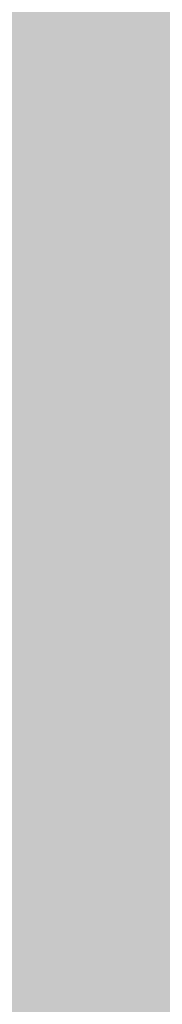
# Model space of a CAD drawing. Units: millimetres. Extents: x -22994 to 29398, y -19990 to 20176.
# Tile 80 of 135: x 225.543 to 225.814, y 85.199 to 87.071. Entities that reach past the tile are written whole.
import ezdxf
from ezdxf import colors
from ezdxf.entities.mleader import LeaderData, LeaderLine
from ezdxf.math import Vec2, Vec3

# ---------------------------------------------------------------- set-up
doc = ezdxf.new("R2010")
doc.units = ezdxf.units.MM
doc.header["$MEASUREMENT"] = 0
doc.layers.add('M-ANNO-TEXT', color=7, linetype='Continuous', lineweight=25)
doc.layers.add('M-DIMS', color=2, linetype='Continuous', lineweight=18)
doc.styles.get("Standard").update_dxf_attribs({"font": 'arial.ttf'})
doc.dimstyles.get("Standard").update_dxf_attribs({"dimtxt": 0.18, "dimasz": 10000, "dimexe": 0.18, "dimexo": 0.0625, "dimgap": 0.09, "dimtad": 0, "dimtih": 1, "dimtoh": 1, "dimdec": 0, "dimzin": 0, "dimdsep": 46, "dimtxsty": 'Standard', "dimcen": 0.09, "dimadec": 0, "dimazin": 0, "dimtfac": 1, "dimtdec": 0, "dimtofl": 0, "dimtmove": 0, "dimatfit": 3, "dimfxl": 1, "dimtolj": 1, "dimtzin": 0, "dimlwd": 30, "dimarcsym": 0})

# ---------------------------------------------------------------- blocks, each defined once
blk = doc.blocks.new('*D2')
at = {"layer": 'Defpoints', "color": 0, "transparency": 16777216}
for p in [(6.6773, 10.2713), (290.852, 10.2713), (290.852, -5.0787)]:
    blk.add_point(p, dxfattribs=at)
at = {"layer": 'M-DIMS', "color": 0, "lineweight": -2, "transparency": 16777216}
for p, q in [((6.6773, 10.2088), (6.6773, -5.2587)), ((290.852, 10.2088), (290.852, -5.2587))]:
    blk.add_line(p, q, dxfattribs=at)
at = {"layer": 'M-DIMS', "color": 0, "lineweight": 30, "transparency": 16777216}
for p, q in [((-9993.3227, -5.0787), (-19993.3227, -5.0787)), ((10290.852, -5.0787), (20290.852, -5.0787))]:
    blk.add_line(p, q, dxfattribs=at)
at = {"layer": 'M-DIMS', "color": 0, "transparency": 16777216}
for points in [[(-9993.3227, 1661.5879), (-9993.3227, -1671.7454), (6.6773, -5.0787)], [(10290.852, 1661.5879), (10290.852, -1671.7454), (290.852, -5.0787)]]:
    blk.add_solid(points, dxfattribs=at)
at = {"layer": 'M-DIMS', "color": 0, "transparency": 16777216, "insert": (148.7647, -5.0787), "char_height": 0.18, "attachment_point": 5}
blk.add_mtext('\\A1;284.2', dxfattribs=at)
blk = doc.blocks.new('*D3')
at = {"layer": 'Defpoints', "color": 0, "transparency": 16777216}
for p in [(110.2647, 204.1654), (110.2647, 176.3662), (95.8327, 127.967)]:
    blk.add_point(p, dxfattribs=at)
at = {"layer": 'M-DIMS', "color": 0, "lineweight": -2, "transparency": 16777216}
for p, q in [((95.8327, 128.0295), (95.8327, 204.3454)), ((110.2647, 176.4287), (110.2647, 204.3454))]:
    blk.add_line(p, q, dxfattribs=at)
at = {"layer": 'M-DIMS', "color": 0, "lineweight": 30, "transparency": 16777216}
for p, q in [((-9904.1673, 204.1654), (-19904.1673, 204.1654)), ((10110.2647, 204.1654), (20110.2647, 204.1654))]:
    blk.add_line(p, q, dxfattribs=at)
at = {"layer": 'M-DIMS', "color": 0, "transparency": 16777216}
for points in [[(-9904.1673, 1870.8321), (-9904.1673, -1462.5013), (95.8327, 204.1654)], [(10110.2647, 1870.8321), (10110.2647, -1462.5013), (110.2647, 204.1654)]]:
    blk.add_solid(points, dxfattribs=at)
at = {"layer": 'M-DIMS', "color": 0, "transparency": 16777216, "insert": (103.0487, 204.1654), "char_height": 0.18, "attachment_point": 5}
blk.add_mtext('\\A1;14.432', dxfattribs=at)
blk = doc.blocks.new('*D4')
at = {"layer": 'Defpoints', "color": 0, "transparency": 16777216}
for p in [(116.2647, 204.1654), (110.2647, 176.3662), (116.2647, 176.3662)]:
    blk.add_point(p, dxfattribs=at)
at = {"layer": 'M-DIMS', "color": 0, "lineweight": -2, "transparency": 16777216}
for p, q in [((110.2647, 176.4287), (110.2647, 204.3454)), ((116.2647, 176.4287), (116.2647, 204.3454))]:
    blk.add_line(p, q, dxfattribs=at)
at = {"layer": 'M-DIMS', "color": 0, "lineweight": 30, "transparency": 16777216}
for p, q in [((-9889.7353, 204.1654), (-19889.7353, 204.1654)), ((10116.2647, 204.1654), (20116.2647, 204.1654))]:
    blk.add_line(p, q, dxfattribs=at)
at = {"layer": 'M-DIMS', "color": 0, "transparency": 16777216}
for points in [[(-9889.7353, 1870.8321), (-9889.7353, -1462.5013), (110.2647, 204.1654)], [(10116.2647, 1870.8321), (10116.2647, -1462.5013), (116.2647, 204.1654)]]:
    blk.add_solid(points, dxfattribs=at)
at = {"layer": 'M-DIMS', "color": 0, "transparency": 16777216, "insert": (113.2647, 204.1654), "char_height": 0.18, "attachment_point": 5}
blk.add_mtext('\\A1;6', dxfattribs=at)
blk = doc.blocks.new('*D5')
at = {"layer": 'Defpoints', "color": 0, "transparency": 16777216}
for p in [(181.2647, 204.1654), (116.2647, 176.3662), (181.2647, 176.3662)]:
    blk.add_point(p, dxfattribs=at)
at = {"layer": 'M-DIMS', "color": 0, "lineweight": -2, "transparency": 16777216}
for p, q in [((116.2647, 176.4287), (116.2647, 204.3454)), ((181.2647, 176.4287), (181.2647, 204.3454))]:
    blk.add_line(p, q, dxfattribs=at)
at = {"layer": 'M-DIMS', "color": 0, "lineweight": 30, "transparency": 16777216}
for p, q in [((-9883.7353, 204.1654), (-19883.7353, 204.1654)), ((10181.2647, 204.1654), (20181.2647, 204.1654))]:
    blk.add_line(p, q, dxfattribs=at)
at = {"layer": 'M-DIMS', "color": 0, "transparency": 16777216}
for points in [[(-9883.7353, 1870.8321), (-9883.7353, -1462.5013), (116.2647, 204.1654)], [(10181.2647, 1870.8321), (10181.2647, -1462.5013), (181.2647, 204.1654)]]:
    blk.add_solid(points, dxfattribs=at)
at = {"layer": 'M-DIMS', "color": 0, "transparency": 16777216, "insert": (148.7647, 204.1654), "char_height": 0.18, "attachment_point": 5}
blk.add_mtext('\\A1;65', dxfattribs=at)
blk = doc.blocks.new('*D6')
at = {"layer": 'Defpoints', "color": 0, "transparency": 16777216}
for p in [(187.2647, 204.1654), (181.2647, 176.3662), (187.2647, 176.3662)]:
    blk.add_point(p, dxfattribs=at)
at = {"layer": 'M-DIMS', "color": 0, "lineweight": -2, "transparency": 16777216}
for p, q in [((181.2647, 176.4287), (181.2647, 204.3454)), ((187.2647, 176.4287), (187.2647, 204.3454))]:
    blk.add_line(p, q, dxfattribs=at)
at = {"layer": 'M-DIMS', "color": 0, "lineweight": 30, "transparency": 16777216}
for p, q in [((-9818.7353, 204.1654), (-19818.7353, 204.1654)), ((10187.2647, 204.1654), (20187.2647, 204.1654))]:
    blk.add_line(p, q, dxfattribs=at)
at = {"layer": 'M-DIMS', "color": 0, "transparency": 16777216}
for points in [[(-9818.7353, 1870.8321), (-9818.7353, -1462.5013), (181.2647, 204.1654)], [(10187.2647, 1870.8321), (10187.2647, -1462.5013), (187.2647, 204.1654)]]:
    blk.add_solid(points, dxfattribs=at)
at = {"layer": 'M-DIMS', "color": 0, "transparency": 16777216, "insert": (184.2647, 204.1654), "char_height": 0.18, "attachment_point": 5}
blk.add_mtext('\\A1;6', dxfattribs=at)
blk = doc.blocks.new('*D7')
at = {"layer": 'Defpoints', "color": 0, "transparency": 16777216}
for p in [(201.6967, 204.1654), (187.2647, 176.3662), (201.6967, 127.967)]:
    blk.add_point(p, dxfattribs=at)
at = {"layer": 'M-DIMS', "color": 0, "lineweight": -2, "transparency": 16777216}
for p, q in [((187.2647, 176.4287), (187.2647, 204.3454)), ((201.6967, 128.0295), (201.6967, 204.3454))]:
    blk.add_line(p, q, dxfattribs=at)
at = {"layer": 'M-DIMS', "color": 0, "lineweight": 30, "transparency": 16777216}
for p, q in [((-9812.7353, 204.1654), (-19812.7353, 204.1654)), ((10201.6967, 204.1654), (20201.6967, 204.1654))]:
    blk.add_line(p, q, dxfattribs=at)
at = {"layer": 'M-DIMS', "color": 0, "transparency": 16777216}
for points in [[(-9812.7353, 1870.8321), (-9812.7353, -1462.5013), (187.2647, 204.1654)], [(10201.6967, 1870.8321), (10201.6967, -1462.5013), (201.6967, 204.1654)]]:
    blk.add_solid(points, dxfattribs=at)
at = {"layer": 'M-DIMS', "color": 0, "transparency": 16777216, "insert": (194.4807, 204.1654), "char_height": 0.18, "attachment_point": 5}
blk.add_mtext('\\A1;14.432', dxfattribs=at)
blk = doc.blocks.new('*D8')
at = {"layer": 'Defpoints', "color": 0, "transparency": 16777216}
for p in [(227.6485, 204.1654), (227.6485, 146.7296), (201.6967, 127.967)]:
    blk.add_point(p, dxfattribs=at)
at = {"layer": 'M-DIMS', "color": 0, "lineweight": -2, "transparency": 16777216}
for p, q in [((201.6967, 128.0295), (201.6967, 204.3454)), ((227.6485, 146.7921), (227.6485, 204.3454))]:
    blk.add_line(p, q, dxfattribs=at)
at = {"layer": 'M-DIMS', "color": 0, "lineweight": 30, "transparency": 16777216}
for p, q in [((-9798.3033, 204.1654), (-19798.3033, 204.1654)), ((10227.6485, 204.1654), (20227.6485, 204.1654))]:
    blk.add_line(p, q, dxfattribs=at)
at = {"layer": 'M-DIMS', "color": 0, "transparency": 16777216}
for points in [[(-9798.3033, 1870.8321), (-9798.3033, -1462.5013), (201.6967, 204.1654)], [(10227.6485, 1870.8321), (10227.6485, -1462.5013), (227.6485, 204.1654)]]:
    blk.add_solid(points, dxfattribs=at)
at = {"layer": 'M-DIMS', "color": 0, "transparency": 16777216, "insert": (214.6726, 204.1654), "char_height": 0.18, "attachment_point": 5}
blk.add_mtext('\\A1;25.95', dxfattribs=at)
blk = doc.blocks.new('*D9')
at = {"layer": 'Defpoints', "color": 0, "transparency": 16777216}
for p in [(187.2647, 176.3662), (306.202, 176.3662), (290.852, 10.2713)]:
    blk.add_point(p, dxfattribs=at)
at = {"layer": 'M-DIMS', "color": 0, "lineweight": 30, "transparency": 16777216}
for p, q in [((306.202, 10176.3662), (306.202, 20176.3662)), ((306.202, -9989.7287), (306.202, -19989.7287))]:
    blk.add_line(p, q, dxfattribs=at)
at = {"layer": 'M-DIMS', "color": 0, "lineweight": -2, "transparency": 16777216}
for p, q in [((187.3272, 176.3662), (306.382, 176.3662)), ((290.9145, 10.2713), (306.382, 10.2713))]:
    blk.add_line(p, q, dxfattribs=at)
at = {"layer": 'M-DIMS', "color": 0, "transparency": 16777216}
for points in [[(-1360.4646, 10176.3662), (1972.8687, 10176.3662), (306.202, 176.3662)], [(-1360.4646, -9989.7287), (1972.8687, -9989.7287), (306.202, 10.2713)]]:
    blk.add_solid(points, dxfattribs=at)
at = {"layer": 'M-DIMS', "color": 0, "transparency": 16777216, "insert": (306.202, 93.3187), "char_height": 0.18, "attachment_point": 5}
blk.add_mtext('\\A1;166.1', dxfattribs=at)
blk = doc.blocks.new('*D10')
at = {"layer": 'Defpoints', "color": 0, "transparency": 16777216}
for p in [(125.6498, 136.0713), (133.3459, 136.0713), (133.3459, -5.0787)]:
    blk.add_point(p, dxfattribs=at)
at = {"layer": 'M-DIMS', "color": 0, "lineweight": -2, "transparency": 16777216}
for p, q in [((125.6498, 136.0088), (125.6498, -5.2587)), ((133.3459, 136.0088), (133.3459, -5.2587))]:
    blk.add_line(p, q, dxfattribs=at)
at = {"layer": 'M-DIMS', "color": 0, "lineweight": 30, "transparency": 16777216}
for p, q in [((-9874.3502, -5.0787), (-19874.3502, -5.0787)), ((10133.3459, -5.0787), (20133.3459, -5.0787))]:
    blk.add_line(p, q, dxfattribs=at)
at = {"layer": 'M-DIMS', "color": 0, "transparency": 16777216}
for points in [[(-9874.3502, 1661.5879), (-9874.3502, -1671.7454), (125.6498, -5.0787)], [(10133.3459, 1661.5879), (10133.3459, -1671.7454), (133.3459, -5.0787)]]:
    blk.add_solid(points, dxfattribs=at)
at = {"layer": 'M-DIMS', "color": 0, "transparency": 16777216, "insert": (129.4978, -5.0787), "char_height": 0.18, "attachment_point": 5}
blk.add_mtext('\\A1;7.696', dxfattribs=at)
blk = doc.blocks.new('*D11')
at = {"layer": 'Defpoints', "color": 0, "transparency": 16777216}
for p in [(133.3459, 136.0713), (135.6498, 136.0713), (135.6498, -5.0787)]:
    blk.add_point(p, dxfattribs=at)
at = {"layer": 'M-DIMS', "color": 0, "lineweight": -2, "transparency": 16777216}
for p, q in [((133.3459, 136.0088), (133.3459, -5.2587)), ((135.6498, 136.0088), (135.6498, -5.2587))]:
    blk.add_line(p, q, dxfattribs=at)
at = {"layer": 'M-DIMS', "color": 0, "lineweight": 30, "transparency": 16777216}
for p, q in [((-9866.6541, -5.0787), (-19866.6541, -5.0787)), ((10135.6498, -5.0787), (20135.6498, -5.0787))]:
    blk.add_line(p, q, dxfattribs=at)
at = {"layer": 'M-DIMS', "color": 0, "transparency": 16777216}
for points in [[(-9866.6541, 1661.5879), (-9866.6541, -1671.7454), (133.3459, -5.0787)], [(10135.6498, 1661.5879), (10135.6498, -1671.7454), (135.6498, -5.0787)]]:
    blk.add_solid(points, dxfattribs=at)
at = {"layer": 'M-DIMS', "color": 0, "transparency": 16777216, "insert": (134.4978, -5.0787), "char_height": 0.18, "attachment_point": 5}
blk.add_mtext('\\A1;2.304', dxfattribs=at)
blk = doc.blocks.new('*D12')
at = {"layer": 'Defpoints', "color": 0, "transparency": 16777216}
for p in [(135.6498, 136.0713), (145.6498, 136.0713), (145.6498, -5.0787)]:
    blk.add_point(p, dxfattribs=at)
at = {"layer": 'M-DIMS', "color": 0, "lineweight": -2, "transparency": 16777216}
for p, q in [((135.6498, 136.0088), (135.6498, -5.2587)), ((145.6498, 136.0088), (145.6498, -5.2587))]:
    blk.add_line(p, q, dxfattribs=at)
at = {"layer": 'M-DIMS', "color": 0, "lineweight": 30, "transparency": 16777216}
for p, q in [((-9864.3502, -5.0787), (-19864.3502, -5.0787)), ((10145.6498, -5.0787), (20145.6498, -5.0787))]:
    blk.add_line(p, q, dxfattribs=at)
at = {"layer": 'M-DIMS', "color": 0, "transparency": 16777216}
for points in [[(-9864.3502, 1661.5879), (-9864.3502, -1671.7454), (135.6498, -5.0787)], [(10145.6498, 1661.5879), (10145.6498, -1671.7454), (145.6498, -5.0787)]]:
    blk.add_solid(points, dxfattribs=at)
at = {"layer": 'M-DIMS', "color": 0, "transparency": 16777216, "insert": (140.6498, -5.0787), "char_height": 0.18, "attachment_point": 5}
blk.add_mtext('\\A1;10', dxfattribs=at)
blk = doc.blocks.new('*D13')
at = {"layer": 'Defpoints', "color": 0, "transparency": 16777216}
for p in [(145.6498, 136.0713), (155.6498, 136.0713), (155.6498, -5.0787)]:
    blk.add_point(p, dxfattribs=at)
at = {"layer": 'M-DIMS', "color": 0, "lineweight": -2, "transparency": 16777216}
for p, q in [((145.6498, 136.0088), (145.6498, -5.2587)), ((155.6498, 136.0088), (155.6498, -5.2587))]:
    blk.add_line(p, q, dxfattribs=at)
at = {"layer": 'M-DIMS', "color": 0, "lineweight": 30, "transparency": 16777216}
for p, q in [((-9854.3502, -5.0787), (-19854.3502, -5.0787)), ((10155.6498, -5.0787), (20155.6498, -5.0787))]:
    blk.add_line(p, q, dxfattribs=at)
at = {"layer": 'M-DIMS', "color": 0, "transparency": 16777216}
for points in [[(-9854.3502, 1661.5879), (-9854.3502, -1671.7454), (145.6498, -5.0787)], [(10155.6498, 1661.5879), (10155.6498, -1671.7454), (155.6498, -5.0787)]]:
    blk.add_solid(points, dxfattribs=at)
at = {"layer": 'M-DIMS', "color": 0, "transparency": 16777216, "insert": (150.6498, -5.0787), "char_height": 0.18, "attachment_point": 5}
blk.add_mtext('\\A1;10', dxfattribs=at)
blk = doc.blocks.new('*D14')
at = {"layer": 'Defpoints', "color": 0, "transparency": 16777216}
for p in [(155.6498, 136.0713), (165.6498, 136.0713), (165.6498, -5.0787)]:
    blk.add_point(p, dxfattribs=at)
at = {"layer": 'M-DIMS', "color": 0, "lineweight": -2, "transparency": 16777216}
for p, q in [((155.6498, 136.0088), (155.6498, -5.2587)), ((165.6498, 136.0088), (165.6498, -5.2587))]:
    blk.add_line(p, q, dxfattribs=at)
at = {"layer": 'M-DIMS', "color": 0, "lineweight": 30, "transparency": 16777216}
for p, q in [((-9844.3502, -5.0787), (-19844.3502, -5.0787)), ((10165.6498, -5.0787), (20165.6498, -5.0787))]:
    blk.add_line(p, q, dxfattribs=at)
at = {"layer": 'M-DIMS', "color": 0, "transparency": 16777216}
for points in [[(-9844.3502, 1661.5879), (-9844.3502, -1671.7454), (155.6498, -5.0787)], [(10165.6498, 1661.5879), (10165.6498, -1671.7454), (165.6498, -5.0787)]]:
    blk.add_solid(points, dxfattribs=at)
at = {"layer": 'M-DIMS', "color": 0, "transparency": 16777216, "insert": (160.6498, -5.0787), "char_height": 0.18, "attachment_point": 5}
blk.add_mtext('\\A1;10', dxfattribs=at)
blk = doc.blocks.new('*D15')
at = {"layer": 'Defpoints', "color": 0, "transparency": 16777216}
for p in [(173.3459, 154.788), (173.3459, 136.0713), (306.202, 136.0713)]:
    blk.add_point(p, dxfattribs=at)
at = {"layer": 'M-DIMS', "color": 0, "lineweight": 30, "transparency": 16777216}
for p, q in [((306.202, 10154.788), (306.202, 20154.788)), ((306.202, -9863.9287), (306.202, -19863.9287))]:
    blk.add_line(p, q, dxfattribs=at)
at = {"layer": 'M-DIMS', "color": 0, "lineweight": -2, "transparency": 16777216}
for p, q in [((173.4084, 154.788), (306.382, 154.788)), ((173.4084, 136.0713), (306.382, 136.0713))]:
    blk.add_line(p, q, dxfattribs=at)
at = {"layer": 'M-DIMS', "color": 0, "transparency": 16777216}
for points in [[(-1360.4646, 10154.788), (1972.8687, 10154.788), (306.202, 154.788)], [(-1360.4646, -9863.9287), (1972.8687, -9863.9287), (306.202, 136.0713)]]:
    blk.add_solid(points, dxfattribs=at)
at = {"layer": 'M-DIMS', "color": 0, "transparency": 16777216, "insert": (306.202, 145.4297), "char_height": 0.18, "attachment_point": 5}
blk.add_mtext('\\A1;18.717', dxfattribs=at)
blk = doc.blocks.new('*D16')
at = {"layer": 'Defpoints', "color": 0, "transparency": 16777216}
for p in [(120.1702, 204.1654), (110.4658, 48.0349), (120.1702, 48.0349)]:
    blk.add_point(p, dxfattribs=at)
at = {"layer": 'M-DIMS', "color": 0, "lineweight": -2, "transparency": 16777216}
for p, q in [((110.4658, 48.0974), (110.4658, 204.3454)), ((120.1702, 48.0974), (120.1702, 204.3454))]:
    blk.add_line(p, q, dxfattribs=at)
at = {"layer": 'M-DIMS', "color": 0, "lineweight": 30, "transparency": 16777216}
for p, q in [((-9889.5342, 204.1654), (-19889.5342, 204.1654)), ((10120.1702, 204.1654), (20120.1702, 204.1654))]:
    blk.add_line(p, q, dxfattribs=at)
at = {"layer": 'M-DIMS', "color": 0, "transparency": 16777216}
for points in [[(-9889.5342, 1870.8321), (-9889.5342, -1462.5013), (110.4658, 204.1654)], [(10120.1702, 1870.8321), (10120.1702, -1462.5013), (120.1702, 204.1654)]]:
    blk.add_solid(points, dxfattribs=at)
at = {"layer": 'M-DIMS', "color": 0, "transparency": 16777216, "insert": (115.318, 204.1654), "char_height": 0.18, "attachment_point": 5}
blk.add_mtext('\\A1;9.704', dxfattribs=at)
blk = doc.blocks.new('*D17')
at = {"layer": 'Defpoints', "color": 0, "transparency": 16777216}
for p in [(126.1702, 204.1654), (120.1702, 48.0349), (126.1702, 48.0349)]:
    blk.add_point(p, dxfattribs=at)
at = {"layer": 'M-DIMS', "color": 0, "lineweight": -2, "transparency": 16777216}
for p, q in [((120.1702, 48.0974), (120.1702, 204.3454)), ((126.1702, 48.0974), (126.1702, 204.3454))]:
    blk.add_line(p, q, dxfattribs=at)
at = {"layer": 'M-DIMS', "color": 0, "lineweight": 30, "transparency": 16777216}
for p, q in [((-9879.8298, 204.1654), (-19879.8298, 204.1654)), ((10126.1702, 204.1654), (20126.1702, 204.1654))]:
    blk.add_line(p, q, dxfattribs=at)
at = {"layer": 'M-DIMS', "color": 0, "transparency": 16777216}
for points in [[(-9879.8298, 1870.8321), (-9879.8298, -1462.5013), (120.1702, 204.1654)], [(10126.1702, 1870.8321), (10126.1702, -1462.5013), (126.1702, 204.1654)]]:
    blk.add_solid(points, dxfattribs=at)
at = {"layer": 'M-DIMS', "color": 0, "transparency": 16777216, "insert": (123.1702, 204.1654), "char_height": 0.18, "attachment_point": 5}
blk.add_mtext('\\A1;6', dxfattribs=at)
blk = doc.blocks.new('*D18')
at = {"layer": 'Defpoints', "color": 0, "transparency": 16777216}
for p in [(132.1702, 204.1654), (126.1702, 48.0349), (132.1702, 48.0349)]:
    blk.add_point(p, dxfattribs=at)
at = {"layer": 'M-DIMS', "color": 0, "lineweight": -2, "transparency": 16777216}
for p, q in [((126.1702, 48.0974), (126.1702, 204.3454)), ((132.1702, 48.0974), (132.1702, 204.3454))]:
    blk.add_line(p, q, dxfattribs=at)
at = {"layer": 'M-DIMS', "color": 0, "lineweight": 30, "transparency": 16777216}
for p, q in [((-9873.8298, 204.1654), (-19873.8298, 204.1654)), ((10132.1702, 204.1654), (20132.1702, 204.1654))]:
    blk.add_line(p, q, dxfattribs=at)
at = {"layer": 'M-DIMS', "color": 0, "transparency": 16777216}
for points in [[(-9873.8298, 1870.8321), (-9873.8298, -1462.5013), (126.1702, 204.1654)], [(10132.1702, 1870.8321), (10132.1702, -1462.5013), (132.1702, 204.1654)]]:
    blk.add_solid(points, dxfattribs=at)
at = {"layer": 'M-DIMS', "color": 0, "transparency": 16777216, "insert": (129.1702, 204.1654), "char_height": 0.18, "attachment_point": 5}
blk.add_mtext('\\A1;6', dxfattribs=at)
blk = doc.blocks.new('*D19')
at = {"layer": 'Defpoints', "color": 0, "transparency": 16777216}
for p in [(138.1702, 204.1654), (132.1702, 48.0349), (138.1702, 48.0349)]:
    blk.add_point(p, dxfattribs=at)
at = {"layer": 'M-DIMS', "color": 0, "lineweight": -2, "transparency": 16777216}
for p, q in [((132.1702, 48.0974), (132.1702, 204.3454)), ((138.1702, 48.0974), (138.1702, 204.3454))]:
    blk.add_line(p, q, dxfattribs=at)
at = {"layer": 'M-DIMS', "color": 0, "lineweight": 30, "transparency": 16777216}
for p, q in [((-9867.8298, 204.1654), (-19867.8298, 204.1654)), ((10138.1702, 204.1654), (20138.1702, 204.1654))]:
    blk.add_line(p, q, dxfattribs=at)
at = {"layer": 'M-DIMS', "color": 0, "transparency": 16777216}
for points in [[(-9867.8298, 1870.8321), (-9867.8298, -1462.5013), (132.1702, 204.1654)], [(10138.1702, 1870.8321), (10138.1702, -1462.5013), (138.1702, 204.1654)]]:
    blk.add_solid(points, dxfattribs=at)
at = {"layer": 'M-DIMS', "color": 0, "transparency": 16777216, "insert": (135.1702, 204.1654), "char_height": 0.18, "attachment_point": 5}
blk.add_mtext('\\A1;6', dxfattribs=at)
blk = doc.blocks.new('*D20')
at = {"layer": 'Defpoints', "color": 0, "transparency": 16777216}
for p in [(144.1702, 204.1654), (138.1702, 48.0349), (144.1702, 48.0349)]:
    blk.add_point(p, dxfattribs=at)
at = {"layer": 'M-DIMS', "color": 0, "lineweight": -2, "transparency": 16777216}
for p, q in [((138.1702, 48.0974), (138.1702, 204.3454)), ((144.1702, 48.0974), (144.1702, 204.3454))]:
    blk.add_line(p, q, dxfattribs=at)
at = {"layer": 'M-DIMS', "color": 0, "lineweight": 30, "transparency": 16777216}
for p, q in [((-9861.8298, 204.1654), (-19861.8298, 204.1654)), ((10144.1702, 204.1654), (20144.1702, 204.1654))]:
    blk.add_line(p, q, dxfattribs=at)
at = {"layer": 'M-DIMS', "color": 0, "transparency": 16777216}
for points in [[(-9861.8298, 1870.8321), (-9861.8298, -1462.5013), (138.1702, 204.1654)], [(10144.1702, 1870.8321), (10144.1702, -1462.5013), (144.1702, 204.1654)]]:
    blk.add_solid(points, dxfattribs=at)
at = {"layer": 'M-DIMS', "color": 0, "transparency": 16777216, "insert": (141.1702, 204.1654), "char_height": 0.18, "attachment_point": 5}
blk.add_mtext('\\A1;6', dxfattribs=at)
blk = doc.blocks.new('*D21')
at = {"layer": 'Defpoints', "color": 0, "transparency": 16777216}
for p in [(149.1157, 204.1654), (144.1702, 48.0349), (149.1157, 48.0349)]:
    blk.add_point(p, dxfattribs=at)
at = {"layer": 'M-DIMS', "color": 0, "lineweight": -2, "transparency": 16777216}
for p, q in [((144.1702, 48.0974), (144.1702, 204.3454)), ((149.1157, 48.0974), (149.1157, 204.3454))]:
    blk.add_line(p, q, dxfattribs=at)
at = {"layer": 'M-DIMS', "color": 0, "lineweight": 30, "transparency": 16777216}
for p, q in [((-9855.8298, 204.1654), (-19855.8298, 204.1654)), ((10149.1157, 204.1654), (20149.1157, 204.1654))]:
    blk.add_line(p, q, dxfattribs=at)
at = {"layer": 'M-DIMS', "color": 0, "transparency": 16777216}
for points in [[(-9855.8298, 1870.8321), (-9855.8298, -1462.5013), (144.1702, 204.1654)], [(10149.1157, 1870.8321), (10149.1157, -1462.5013), (149.1157, 204.1654)]]:
    blk.add_solid(points, dxfattribs=at)
at = {"layer": 'M-DIMS', "color": 0, "transparency": 16777216, "insert": (146.6429, 204.1654), "char_height": 0.18, "attachment_point": 5}
blk.add_mtext('\\A1;4.945', dxfattribs=at)
blk = doc.blocks.new('*D22')
at = {"layer": 'Defpoints', "color": 0, "transparency": 16777216}
for p in [(149.1157, 30.9895), (155.1157, 30.9895), (155.1157, -5.0787)]:
    blk.add_point(p, dxfattribs=at)
at = {"layer": 'M-DIMS', "color": 0, "lineweight": -2, "transparency": 16777216}
for p, q in [((149.1157, 30.927), (149.1157, -5.2587)), ((155.1157, 30.927), (155.1157, -5.2587))]:
    blk.add_line(p, q, dxfattribs=at)
at = {"layer": 'M-DIMS', "color": 0, "lineweight": 30, "transparency": 16777216}
for p, q in [((-9850.8843, -5.0787), (-19850.8843, -5.0787)), ((10155.1157, -5.0787), (20155.1157, -5.0787))]:
    blk.add_line(p, q, dxfattribs=at)
at = {"layer": 'M-DIMS', "color": 0, "transparency": 16777216}
for points in [[(-9850.8843, 1661.5879), (-9850.8843, -1671.7454), (149.1157, -5.0787)], [(10155.1157, 1661.5879), (10155.1157, -1671.7454), (155.1157, -5.0787)]]:
    blk.add_solid(points, dxfattribs=at)
at = {"layer": 'M-DIMS', "color": 0, "transparency": 16777216, "insert": (152.1157, -5.0787), "char_height": 0.18, "attachment_point": 5}
blk.add_mtext('\\A1;6', dxfattribs=at)
blk = doc.blocks.new('*D23')
at = {"layer": 'Defpoints', "color": 0, "transparency": 16777216}
for p in [(155.1157, 30.9895), (161.1157, 30.9895), (161.1157, -5.0787)]:
    blk.add_point(p, dxfattribs=at)
at = {"layer": 'M-DIMS', "color": 0, "lineweight": -2, "transparency": 16777216}
for p, q in [((155.1157, 30.927), (155.1157, -5.2587)), ((161.1157, 30.927), (161.1157, -5.2587))]:
    blk.add_line(p, q, dxfattribs=at)
at = {"layer": 'M-DIMS', "color": 0, "lineweight": 30, "transparency": 16777216}
for p, q in [((-9844.8843, -5.0787), (-19844.8843, -5.0787)), ((10161.1157, -5.0787), (20161.1157, -5.0787))]:
    blk.add_line(p, q, dxfattribs=at)
at = {"layer": 'M-DIMS', "color": 0, "transparency": 16777216}
for points in [[(-9844.8843, 1661.5879), (-9844.8843, -1671.7454), (155.1157, -5.0787)], [(10161.1157, 1661.5879), (10161.1157, -1671.7454), (161.1157, -5.0787)]]:
    blk.add_solid(points, dxfattribs=at)
at = {"layer": 'M-DIMS', "color": 0, "transparency": 16777216, "insert": (158.1157, -5.0787), "char_height": 0.18, "attachment_point": 5}
blk.add_mtext('\\A1;6', dxfattribs=at)
blk = doc.blocks.new('*D24')
at = {"layer": 'Defpoints', "color": 0, "transparency": 16777216}
for p in [(161.1157, 30.9895), (166.4387, 30.9895), (166.4387, -5.0787)]:
    blk.add_point(p, dxfattribs=at)
at = {"layer": 'M-DIMS', "color": 0, "lineweight": -2, "transparency": 16777216}
for p, q in [((161.1157, 30.927), (161.1157, -5.2587)), ((166.4387, 30.927), (166.4387, -5.2587))]:
    blk.add_line(p, q, dxfattribs=at)
at = {"layer": 'M-DIMS', "color": 0, "lineweight": 30, "transparency": 16777216}
for p, q in [((-9838.8843, -5.0787), (-19838.8843, -5.0787)), ((10166.4387, -5.0787), (20166.4387, -5.0787))]:
    blk.add_line(p, q, dxfattribs=at)
at = {"layer": 'M-DIMS', "color": 0, "transparency": 16777216}
for points in [[(-9838.8843, 1661.5879), (-9838.8843, -1671.7454), (161.1157, -5.0787)], [(10166.4387, 1661.5879), (10166.4387, -1671.7454), (166.4387, -5.0787)]]:
    blk.add_solid(points, dxfattribs=at)
at = {"layer": 'M-DIMS', "color": 0, "transparency": 16777216, "insert": (163.7772, -5.0787), "char_height": 0.18, "attachment_point": 5}
blk.add_mtext('\\A1;5.323', dxfattribs=at)
blk = doc.blocks.new('*D25')
at = {"layer": 'Defpoints', "color": 0, "transparency": 16777216}
for p in [(166.4387, 30.9895), (172.4387, 30.9895), (172.4387, -5.0787)]:
    blk.add_point(p, dxfattribs=at)
at = {"layer": 'M-DIMS', "color": 0, "lineweight": -2, "transparency": 16777216}
for p, q in [((166.4387, 30.927), (166.4387, -5.2587)), ((172.4387, 30.927), (172.4387, -5.2587))]:
    blk.add_line(p, q, dxfattribs=at)
at = {"layer": 'M-DIMS', "color": 0, "lineweight": 30, "transparency": 16777216}
for p, q in [((-9833.5613, -5.0787), (-19833.5613, -5.0787)), ((10172.4387, -5.0787), (20172.4387, -5.0787))]:
    blk.add_line(p, q, dxfattribs=at)
at = {"layer": 'M-DIMS', "color": 0, "transparency": 16777216}
for points in [[(-9833.5613, 1661.5879), (-9833.5613, -1671.7454), (166.4387, -5.0787)], [(10172.4387, 1661.5879), (10172.4387, -1671.7454), (172.4387, -5.0787)]]:
    blk.add_solid(points, dxfattribs=at)
at = {"layer": 'M-DIMS', "color": 0, "transparency": 16777216, "insert": (169.4387, -5.0787), "char_height": 0.18, "attachment_point": 5}
blk.add_mtext('\\A1;6', dxfattribs=at)
blk = doc.blocks.new('*D26')
at = {"layer": 'Defpoints', "color": 0, "transparency": 16777216}
for p in [(172.4387, 30.9895), (178.4387, 30.9895), (178.4387, -5.0787)]:
    blk.add_point(p, dxfattribs=at)
at = {"layer": 'M-DIMS', "color": 0, "lineweight": -2, "transparency": 16777216}
for p, q in [((172.4387, 30.927), (172.4387, -5.2587)), ((178.4387, 30.927), (178.4387, -5.2587))]:
    blk.add_line(p, q, dxfattribs=at)
at = {"layer": 'M-DIMS', "color": 0, "lineweight": 30, "transparency": 16777216}
for p, q in [((-9827.5613, -5.0787), (-19827.5613, -5.0787)), ((10178.4387, -5.0787), (20178.4387, -5.0787))]:
    blk.add_line(p, q, dxfattribs=at)
at = {"layer": 'M-DIMS', "color": 0, "transparency": 16777216}
for points in [[(-9827.5613, 1661.5879), (-9827.5613, -1671.7454), (172.4387, -5.0787)], [(10178.4387, 1661.5879), (10178.4387, -1671.7454), (178.4387, -5.0787)]]:
    blk.add_solid(points, dxfattribs=at)
at = {"layer": 'M-DIMS', "color": 0, "transparency": 16777216, "insert": (175.4387, -5.0787), "char_height": 0.18, "attachment_point": 5}
blk.add_mtext('\\A1;6', dxfattribs=at)
blk = doc.blocks.new('*D27')
at = {"layer": 'Defpoints', "color": 0, "transparency": 16777216}
for p in [(178.4387, 30.9895), (188.1175, 30.9895), (188.1175, -5.0787)]:
    blk.add_point(p, dxfattribs=at)
at = {"layer": 'M-DIMS', "color": 0, "lineweight": -2, "transparency": 16777216}
for p, q in [((178.4387, 30.927), (178.4387, -5.2587)), ((188.1175, 30.927), (188.1175, -5.2587))]:
    blk.add_line(p, q, dxfattribs=at)
at = {"layer": 'M-DIMS', "color": 0, "lineweight": 30, "transparency": 16777216}
for p, q in [((-9821.5613, -5.0787), (-19821.5613, -5.0787)), ((10188.1175, -5.0787), (20188.1175, -5.0787))]:
    blk.add_line(p, q, dxfattribs=at)
at = {"layer": 'M-DIMS', "color": 0, "transparency": 16777216}
for points in [[(-9821.5613, 1661.5879), (-9821.5613, -1671.7454), (178.4387, -5.0787)], [(10188.1175, 1661.5879), (10188.1175, -1671.7454), (188.1175, -5.0787)]]:
    blk.add_solid(points, dxfattribs=at)
at = {"layer": 'M-DIMS', "color": 0, "transparency": 16777216, "insert": (183.2781, -5.0787), "char_height": 0.18, "attachment_point": 5}
blk.add_mtext('\\A1;9.679', dxfattribs=at)
blk = doc.blocks.new('*D28')
at = {"layer": 'Defpoints', "color": 0, "transparency": 16777216}
for p in [(188.1175, 48.0349), (306.202, 48.0349), (188.1175, 30.9895)]:
    blk.add_point(p, dxfattribs=at)
at = {"layer": 'M-DIMS', "color": 0, "lineweight": 30, "transparency": 16777216}
for p, q in [((306.202, 10048.0349), (306.202, 20048.0349)), ((306.202, -9969.0105), (306.202, -19969.0105))]:
    blk.add_line(p, q, dxfattribs=at)
at = {"layer": 'M-DIMS', "color": 0, "lineweight": -2, "transparency": 16777216}
for p, q in [((188.18, 48.0349), (306.382, 48.0349)), ((188.18, 30.9895), (306.382, 30.9895))]:
    blk.add_line(p, q, dxfattribs=at)
at = {"layer": 'M-DIMS', "color": 0, "transparency": 16777216}
for points in [[(-1360.4646, 10048.0349), (1972.8687, 10048.0349), (306.202, 48.0349)], [(-1360.4646, -9969.0105), (1972.8687, -9969.0105), (306.202, 30.9895)]]:
    blk.add_solid(points, dxfattribs=at)
at = {"layer": 'M-DIMS', "color": 0, "transparency": 16777216, "insert": (306.202, 39.5122), "char_height": 0.18, "attachment_point": 5}
blk.add_mtext('\\A1;17.045', dxfattribs=at)
blk = doc.blocks.new('*D29')
at = {"layer": 'Defpoints', "color": 0, "transparency": 16777216}
for p in [(36.8006, 80.045), (64.0296, 80.045)]:
    blk.add_point(p, dxfattribs=at)
at = {"layer": 'M-DIMS', "color": 0, "lineweight": -2, "transparency": 16777216}
for p, q in [((50.4151, 79.955), (50.4151, 80.135)), ((50.3251, 80.045), (50.5051, 80.045))]:
    blk.add_line(p, q, dxfattribs=at)
at = {"layer": 'M-DIMS', "color": 0, "lineweight": 30, "transparency": 16777216}
blk.add_line((20064.0296, 80.0303), (10064.0296, 80.0377), dxfattribs=at)
at = {"layer": 'M-DIMS', "color": 0, "transparency": 16777216}
blk.add_solid([(10064.0309, 1746.7043), (10064.0284, -1586.629), (64.0296, 80.045)], dxfattribs=at)
at = {"layer": 'M-DIMS', "color": 0, "transparency": 16777216, "insert": (20064.5213, 80.0303), "char_height": 0.18, "attachment_point": 5}
blk.add_mtext('\\A1;∅27.23', dxfattribs=at)
blk = doc.blocks.new('*D30')
at = {"layer": 'Defpoints', "color": 0, "transparency": 16777216}
for p in [(216.3148, 146.7291), (238.9821, 146.73)]:
    blk.add_point(p, dxfattribs=at)
at = {"layer": 'M-DIMS', "color": 0, "lineweight": 30, "transparency": 16777216}
blk.add_line((20238.9821, 147.4959), (10238.9821, 147.1129), dxfattribs=at)
at = {"layer": 'M-DIMS', "color": 0, "lineweight": -2, "transparency": 16777216}
for p, q in [((227.6485, 146.6396), (227.6485, 146.8196)), ((227.5585, 146.7296), (227.7385, 146.7296))]:
    blk.add_line(p, q, dxfattribs=at)
at = {"layer": 'M-DIMS', "color": 0, "transparency": 16777216}
blk.add_solid([(10238.9183, 1813.7796), (10239.0459, -1519.5537), (238.9821, 146.73)], dxfattribs=at)
at = {"layer": 'M-DIMS', "color": 0, "transparency": 16777216, "insert": (20239.5436, 147.4959), "char_height": 0.18, "attachment_point": 5}
blk.add_mtext('\\A1;∅22.667', dxfattribs=at)
blk = doc.blocks.new('*D31')
at = {"layer": 'Defpoints', "color": 0, "transparency": 16777216}
for p in [(223.1641, 146.7291), (232.1328, 146.73)]:
    blk.add_point(p, dxfattribs=at)
at = {"layer": 'M-DIMS', "color": 0, "lineweight": 30, "transparency": 16777216}
blk.add_line((20232.1327, 148.6656), (10232.1328, 147.6978), dxfattribs=at)
at = {"layer": 'M-DIMS', "color": 0, "lineweight": -2, "transparency": 16777216}
for p, q in [((227.6485, 146.6396), (227.6485, 146.8196)), ((227.5585, 146.7296), (227.7385, 146.7296))]:
    blk.add_line(p, q, dxfattribs=at)
at = {"layer": 'M-DIMS', "color": 0, "transparency": 16777216}
blk.add_solid([(10231.9715, 1814.3645), (10232.2941, -1518.9688), (232.1328, 146.73)], dxfattribs=at)
at = {"layer": 'M-DIMS', "color": 0, "transparency": 16777216, "insert": (20232.6245, 148.6656), "char_height": 0.18, "attachment_point": 5}
blk.add_mtext('\\A1;∅8.969', dxfattribs=at)
blk = doc.blocks.new('*D36')
at = {"layer": 'Defpoints', "color": 0, "transparency": 16777216}
for p in [(46.39, 31.3035), (46.3875, 26.5934)]:
    blk.add_point(p, dxfattribs=at)
at = {"layer": 'M-DIMS', "color": 0, "lineweight": 30, "transparency": 16777216}
for p, q in [((57.1499, 20031.3006), (51.77, 10031.302)), ((10057.1499, 20031.3006), (57.1499, 20031.3006))]:
    blk.add_line(p, q, dxfattribs=at)
at = {"layer": 'M-DIMS', "color": 0, "lineweight": -2, "transparency": 16777216}
for p, q in [((46.3887, 28.8585), (46.3887, 29.0385)), ((46.2987, 28.9485), (46.4787, 28.9485))]:
    blk.add_line(p, q, dxfattribs=at)
at = {"layer": 'M-DIMS', "color": 0, "transparency": 16777216}
blk.add_solid([(-1614.8965, 10032.1987), (1718.4364, 10030.4054), (46.39, 31.3035)], dxfattribs=at)
at = {"layer": 'M-DIMS', "color": 0, "transparency": 16777216, "insert": (10057.5542, 20031.3006), "char_height": 0.18, "attachment_point": 5}
blk.add_mtext('\\A1;∅4.71', dxfattribs=at)
blk = doc.blocks.new('*D37')
at = {"layer": 'Defpoints', "color": 0, "transparency": 16777216}
for p in [(54.8343, 118.6145), (59.4936, 118.614)]:
    blk.add_point(p, dxfattribs=at)
at = {"layer": 'M-DIMS', "color": 0, "lineweight": -2, "transparency": 16777216}
for p, q in [((57.1639, 118.5243), (57.1639, 118.7043)), ((57.0739, 118.6143), (57.2539, 118.6143))]:
    blk.add_line(p, q, dxfattribs=at)
at = {"layer": 'M-DIMS', "color": 0, "lineweight": 30, "transparency": 16777216}
blk.add_line((20059.4934, 116.2531), (10059.4935, 117.4336), dxfattribs=at)
at = {"layer": 'M-DIMS', "color": 0, "transparency": 16777216}
blk.add_solid([(10059.6902, 1784.1002), (10059.2968, -1549.2331), (59.4936, 118.614)], dxfattribs=at)
at = {"layer": 'M-DIMS', "color": 0, "transparency": 16777216, "insert": (20059.9852, 116.2531), "char_height": 0.18, "attachment_point": 5}
blk.add_mtext('\\A1;∅4.659', dxfattribs=at)

msp = doc.modelspace()

# ---------------------------------------------------------------- dimensions: what is measured, and where the dimension line sits
at = {"layer": 'M-DIMS'}
for base, p1, p2, override, picture, middle in [((306.202, 176.3662), (290.852, 10.2713), (187.2647, 176.3662), {"dimdec": 1, "dimlfac": 1, "dimrnd": 0, "dimzin": 0, "dimdsep": 46, "dimlunit": 2}, '*D9', (306.202, 93.3187)), ((306.202, 136.0713), (173.3459, 154.788), (173.3459, 136.0713), {"dimdec": 3, "dimlfac": 1, "dimrnd": 0, "dimzin": 0, "dimdsep": 46, "dimlunit": 2}, '*D15', (306.202, 145.4297)), ((306.202, 48.0349), (188.1175, 30.9895), (188.1175, 48.0349), {"dimdec": 3, "dimlfac": 1, "dimrnd": 0, "dimzin": 0, "dimdsep": 46, "dimlunit": 2}, '*D28', (306.202, 39.5122))]:
    dim = msp.add_linear_dim(base=base, p1=p1, p2=p2, angle=90, dimstyle='Standard', override=override, dxfattribs=at)
    dim.commit()
    dim.dimension.update_dxf_attribs({"geometry": picture, "text_midpoint": middle})
for p1, p2, override, picture, middle in [((46.3875, 26.5934), (46.39, 31.3035), {"dimdec": 2, "dimlfac": 1, "dimrnd": 0, "dimzin": 0, "dimdsep": 46, "dimlunit": 2}, '*D36', (10057.5542, 20031.3006)), ((223.1641, 146.7291), (232.1328, 146.73), {"dimdec": 3, "dimlfac": 1, "dimrnd": 0, "dimzin": 0, "dimdsep": 46, "dimlunit": 2}, '*D31', (20232.1327, 148.6656)), ((216.3148, 146.7291), (238.9821, 146.73), {"dimdec": 3, "dimlfac": 1, "dimrnd": 0, "dimzin": 0, "dimdsep": 46, "dimlunit": 2}, '*D30', (20238.9821, 147.4959))]:
    dim = msp.add_diameter_dim_2p(p1=p1, p2=p2, dimstyle='Standard', override=override, dxfattribs=at)
    dim.commit()
    dim.dimension.update_dxf_attribs({"geometry": picture, "text_midpoint": middle, "dimtype": 163})
for base, p1, p2, override, picture, middle in [((110.2647, 204.1654), (95.8327, 127.967), (110.2647, 176.3662), {"dimdec": 3, "dimlfac": 1, "dimrnd": 0, "dimzin": 0, "dimdsep": 46, "dimlunit": 2}, '*D3', (103.0487, 204.1654)), ((116.2647, 204.1654), (110.2647, 176.3662), (116.2647, 176.3662), {"dimdec": 0, "dimlfac": 1, "dimrnd": 0, "dimzin": 0, "dimdsep": 46, "dimlunit": 2}, '*D4', (113.2647, 204.1654)), ((120.1702, 204.1654), (110.4658, 48.0349), (120.1702, 48.0349), {"dimdec": 3, "dimlfac": 1, "dimrnd": 0, "dimzin": 0, "dimdsep": 46, "dimlunit": 2}, '*D16', (115.318, 204.1654)), ((181.2647, 204.1654), (116.2647, 176.3662), (181.2647, 176.3662), {"dimdec": 0, "dimlfac": 1, "dimrnd": 0, "dimzin": 0, "dimdsep": 46, "dimlunit": 2}, '*D5', (148.7647, 204.1654)), ((126.1702, 204.1654), (120.1702, 48.0349), (126.1702, 48.0349), {"dimdec": 0, "dimlfac": 1, "dimrnd": 0, "dimzin": 0, "dimdsep": 46, "dimlunit": 2}, '*D17', (123.1702, 204.1654)), ((132.1702, 204.1654), (126.1702, 48.0349), (132.1702, 48.0349), {"dimdec": 0, "dimlfac": 1, "dimrnd": 0, "dimzin": 0, "dimdsep": 46, "dimlunit": 2}, '*D18', (129.1702, 204.1654)), ((138.1702, 204.1654), (132.1702, 48.0349), (138.1702, 48.0349), {"dimdec": 0, "dimlfac": 1, "dimrnd": 0, "dimzin": 0, "dimdsep": 46, "dimlunit": 2}, '*D19', (135.1702, 204.1654)), ((144.1702, 204.1654), (138.1702, 48.0349), (144.1702, 48.0349), {"dimdec": 0, "dimlfac": 1, "dimrnd": 0, "dimzin": 0, "dimdsep": 46, "dimlunit": 2}, '*D20', (141.1702, 204.1654)), ((149.11567, 204.16539), (144.17023, 48.03494), (149.11567, 48.03494), {"dimdec": 3, "dimlfac": 1, "dimrnd": 0, "dimzin": 0, "dimdsep": 46, "dimlunit": 2}, '*D21', (146.64295, 204.16539)), ((187.2647, 204.1654), (181.2647, 176.3662), (187.2647, 176.3662), {"dimdec": 0, "dimlfac": 1, "dimrnd": 0, "dimzin": 0, "dimdsep": 46, "dimlunit": 2}, '*D6', (184.2647, 204.1654)), ((201.6967, 204.1654), (187.2647, 176.3662), (201.6967, 127.967), {"dimdec": 3, "dimlfac": 1, "dimrnd": 0, "dimzin": 0, "dimdsep": 46, "dimlunit": 2}, '*D7', (194.4807, 204.1654)), ((227.6485, 204.1654), (201.6967, 127.967), (227.6485, 146.7296), {"dimdec": 2, "dimlfac": 1, "dimrnd": 0, "dimzin": 0, "dimdsep": 46, "dimlunit": 2}, '*D8', (214.6726, 204.1654)), ((290.852, -5.0787), (6.6773, 10.2713), (290.852, 10.2713), {"dimdec": 1, "dimlfac": 1, "dimrnd": 0, "dimzin": 0, "dimdsep": 46, "dimlunit": 2}, '*D2', (148.7647, -5.0787)), ((133.3459, -5.0787), (125.6498, 136.0713), (133.3459, 136.0713), {"dimdec": 3, "dimlfac": 1, "dimrnd": 0, "dimzin": 0, "dimdsep": 46, "dimlunit": 2}, '*D10', (129.4978, -5.0787)), ((135.6498, -5.0787), (133.3459, 136.0713), (135.6498, 136.0713), {"dimdec": 3, "dimlfac": 1, "dimrnd": 0, "dimzin": 0, "dimdsep": 46, "dimlunit": 2}, '*D11', (134.4978, -5.0787)), ((145.6498, -5.0787), (135.6498, 136.0713), (145.6498, 136.0713), {"dimdec": 0, "dimlfac": 1, "dimrnd": 0, "dimzin": 0, "dimdsep": 46, "dimlunit": 2}, '*D12', (140.6498, -5.0787)), ((155.6498, -5.0787), (145.6498, 136.0713), (155.6498, 136.0713), {"dimdec": 0, "dimlfac": 1, "dimrnd": 0, "dimzin": 0, "dimdsep": 46, "dimlunit": 2}, '*D13', (150.6498, -5.0787)), ((155.1157, -5.0787), (149.1157, 30.9895), (155.1157, 30.9895), {"dimdec": 0, "dimlfac": 1, "dimrnd": 0, "dimzin": 0, "dimdsep": 46, "dimlunit": 2}, '*D22', (152.1157, -5.0787)), ((161.1157, -5.0787), (155.1157, 30.9895), (161.1157, 30.9895), {"dimdec": 0, "dimlfac": 1, "dimrnd": 0, "dimzin": 0, "dimdsep": 46, "dimlunit": 2}, '*D23', (158.1157, -5.0787)), ((165.6498, -5.0787), (155.6498, 136.0713), (165.6498, 136.0713), {"dimdec": 0, "dimlfac": 1, "dimrnd": 0, "dimzin": 0, "dimdsep": 46, "dimlunit": 2}, '*D14', (160.6498, -5.0787)), ((166.4387, -5.0787), (161.1157, 30.9895), (166.4387, 30.9895), {"dimdec": 3, "dimlfac": 1, "dimrnd": 0, "dimzin": 0, "dimdsep": 46, "dimlunit": 2}, '*D24', (163.7772, -5.0787)), ((172.4387, -5.0787), (166.4387, 30.9895), (172.4387, 30.9895), {"dimdec": 0, "dimlfac": 1, "dimrnd": 0, "dimzin": 0, "dimdsep": 46, "dimlunit": 2}, '*D25', (169.4387, -5.0787)), ((178.4387, -5.0787), (172.4387, 30.9895), (178.4387, 30.9895), {"dimdec": 0, "dimlfac": 1, "dimrnd": 0, "dimzin": 0, "dimdsep": 46, "dimlunit": 2}, '*D26', (175.4387, -5.0787)), ((188.1175, -5.0787), (178.4387, 30.9895), (188.1175, 30.9895), {"dimdec": 3, "dimlfac": 1, "dimrnd": 0, "dimzin": 0, "dimdsep": 46, "dimlunit": 2}, '*D27', (183.2781, -5.0787))]:
    dim = msp.add_linear_dim(base=base, p1=p1, p2=p2, dimstyle='Standard', override=override, dxfattribs=at)
    dim.commit()
    dim.dimension.update_dxf_attribs({"geometry": picture, "text_midpoint": middle})
for p1, p2, override, picture, middle in [((54.8343, 118.6145), (59.4936, 118.614), {"dimdec": 3, "dimlfac": 1, "dimrnd": 0, "dimzin": 0, "dimdsep": 46, "dimlunit": 2}, '*D37', (20059.4934, 116.2531)), ((36.8006, 80.045), (64.0296, 80.045), {"dimdec": 2, "dimlfac": 1, "dimrnd": 0, "dimzin": 0, "dimdsep": 46, "dimlunit": 2}, '*D29', (20064.0296, 80.0303))]:
    dim = msp.add_diameter_dim_2p(p1=p1, p2=p2, dimstyle='Standard', override=override, dxfattribs=at)
    dim.commit()
    dim.dimension.update_dxf_attribs({"geometry": picture, "text_midpoint": middle})

# ---------------------------------------------------------------- leaders
at = {"layer": 'M-ANNO-TEXT'}
ml = msp.add_multileader_mtext('Standard', dxfattribs=at)
ml.set_content('combustion chamber', color=256)
ml.set_leader_properties()
ml.build(insert=Vec2(0, 0))
ml.multileader.update_dxf_attribs({"dogleg_length": 0.36, "arrow_head_size": 200})
ctx = ml.context
ctx.base_point, ctx.char_height, ctx.arrow_head_size, ctx.landing_gap_size, ctx.plane_origin = Vec3(215.7321, 57.9149), 3, 200, 0.09, Vec3(189.1175, 57.9149)
notes = []
notes.append((ctx, [(0, (1, 1, 0), (215.3721, 57.9149), (1, 0), 0.36, [(0, [(189.1175, 57.9149)], 0, [])])]))
ctx.mtext.insert, ctx.mtext.flow_direction = Vec3(215.8221, 59.4394), 5
for ctx, leaders in notes:
    for number, flags, end, landing, length, lines in leaders:
        leader = LeaderData()
        leader.index, (leader.has_last_leader_line, leader.has_dogleg_vector, leader.attachment_direction) = number, flags
        leader.last_leader_point, leader.dogleg_vector, leader.dogleg_length = Vec3(end), Vec3(landing), length
        for number, points, colour, breaks in lines:
            line = LeaderLine()
            line.index, line.vertices, line.color, line.breaks = number, Vec3.list(points), colors.encode_raw_color(colour), breaks
            leader.lines.append(line)
        ctx.leaders.append(leader)

doc.saveas('drawing.dxf')
